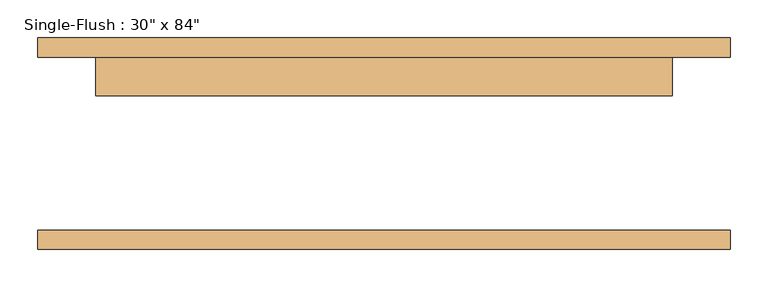
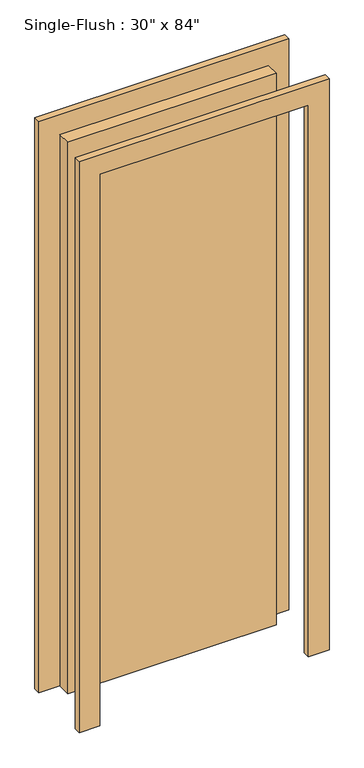
"""IFC4 building model written with IfcOpenShell, lengths in millimetres: door geometry."""

from ifc_helpers import new_model, si_unit, frame, origin, origin_with_axes, place, context, project, spatial, polyline, outline, extrude, source, transform, mapped, element, save


def door_bb98abfd(model_context):
    return source(origin(), model_context, "Body", "SweptSolid", [
        extrude(outline(polyline([(2209.8, -457.2), (0.0, -457.2), (0.0, -381.0), (2133.6, -381.0), (2133.6, 381.0), (0.0, 381.0), (0.0, 457.2), (2209.8, 457.2), (2209.8, -457.2)])), frame((0.0, 114.3, 0.0), z_axis=(0.0, 1.0, 0.0), x_axis=(0.0, 0.0, 1.0)), (0.0, 0.0, 1.0), 25.4),
        extrude(outline(polyline([(2209.8, 457.2), (2209.8, -457.2), (0.0, -457.2), (0.0, -381.0), (2133.6, -381.0), (2133.6, 381.0), (0.0, 381.0), (0.0, 457.2), (2209.8, 457.2)])), frame((0.0, -139.7, 0.0), z_axis=(0.0, 1.0, 0.0), x_axis=(0.0, 0.0, 1.0)), (0.0, 0.0, 1.0), 25.4),
        extrude(outline(polyline([(381.0, 63.5), (-381.0, 63.5), (-381.0, 114.3), (381.0, 114.3), (381.0, 63.5)])), origin_with_axes(), (0.0, 0.0, 1.0), 2133.6),
    ])


if __name__ == "__main__":
    model = new_model("IFC4")
    model_context = context("Model", 3, world=origin())
    ifc_project = project(units=[si_unit("LENGTHUNIT", "METRE", prefix="MILLI")], contexts=[model_context])
    site = spatial("IfcSite", under=ifc_project)
    building = spatial("IfcBuilding", under=site)
    placement = place(None, origin())
    door_shape = door_bb98abfd(model_context)
    element("IfcDoor", 1, ObjectType="Single-Flush : 30\" x 84\"", at=placement, inside=building, context=model_context, shape_type="MappedRepresentation", body=[
        mapped(door_shape, transform((0.0, 0.0, 0.0), x_axis=(1.0, 0.0, 0.0), y_axis=(0.0, 1.0, 0.0), z_axis=(0.0, 0.0, 1.0))),
    ])
    save(model, "model.ifc")

# Revit data of these elements
# Type "Single-Flush : 30\" x 84\""
#   Type Mark = "4"
#   Construction Type Id = "MDOOR"
#   Assembly Code = "C1020"
#   Analytic Construction = "Metal"
#   Thickness = 0.166667 ft
#   Heat Transfer Coefficient (U) = 0.651978 BTU/(h·ft²·°F)
#   Height = 7 ft
#   Trim Projection Ext = 0.083333 ft
#   Trim Projection Int = 0.083333 ft
#   Trim Width = 0.25 ft
#   Width = 2.5 ft
#   Define Thermal Properties by = 1
#   Define Thermal Properties by = 1
#   Door Material = Door - Panel
#   Frame Material = Door - Frame
#   Visual Light Transmittance = 0
#   Solar Heat Gain Coefficient = 0
#   Function = (empty or 0)
#   Wall Closure = (empty or 0)
# Element 1 (IfcDoor, "Single-Flush : 30\" x 84\"")
#   Materials on its faces: "Door - Frame", "Door - Panel"
# Materials
#   "Door - Panel": class "Wood", colour RGB 210 159 95, transparency 0, Cost = 0
#   "Door - Frame": colour RGB 118 70 51, transparency 0, Cost = 0
